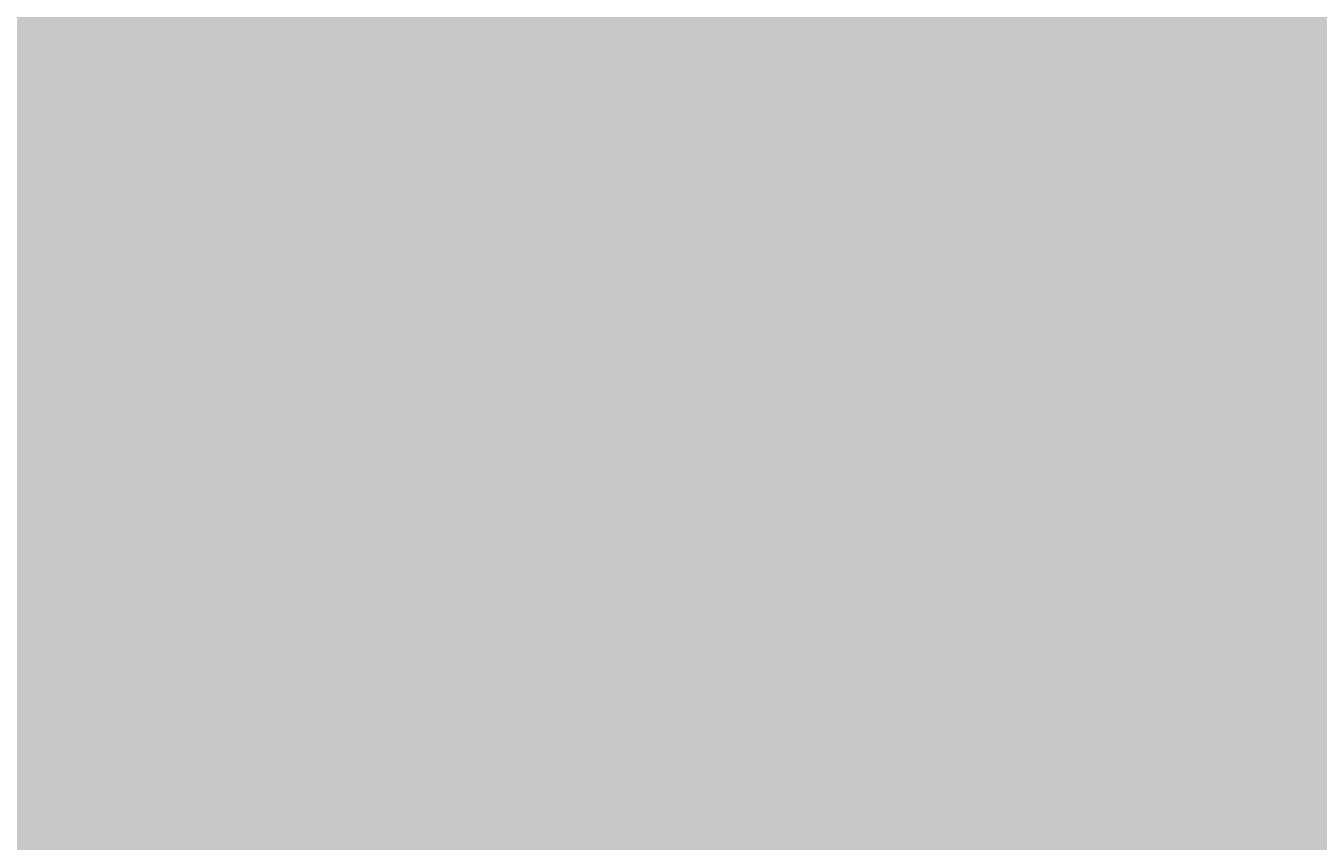
# Model space of a CAD drawing. Units: inches. Extents: x 84 to 1044, y -280 to 906.
# Tile 72 of 105: x 705 to 733, y 432 to 450. Entities that reach past the tile are written whole.
import ezdxf

# ---------------------------------------------------------------- set-up
doc = ezdxf.new("R2010")
doc.units = ezdxf.units.IN
doc.layers.add('A-ANNO-DIMS', color=2, linetype='Continuous', lineweight=18)
doc.layers.add('L-PLNT-PATT', color=9, linetype='Continuous', lineweight=9, true_color=0xafd9aa)
doc.styles.get("Standard").update_dxf_attribs({"font": 'arial.ttf'})
doc.dimstyles.get("Standard").update_dxf_attribs({"dimtxt": 0.18, "dimasz": 0.18, "dimexe": 0.18, "dimexo": 0.0625, "dimgap": 0.09, "dimtad": 0, "dimtih": 1, "dimtoh": 1, "dimdec": 4, "dimzin": 0, "dimdsep": 46, "dimtxsty": 'Standard', "dimcen": 0.09, "dimadec": 0, "dimazin": 0, "dimtfac": 1, "dimtdec": 4, "dimtofl": 0, "dimtmove": 0, "dimatfit": 3, "dimfxl": 1, "dimtolj": 1, "dimtzin": 0, "dimarcsym": 0})

# ---------------------------------------------------------------- blocks, each defined once
blk = doc.blocks.new('*D62')
at = {"layer": 'A-ANNO-DIMS', "color": 0, "lineweight": -2, "transparency": 16777216}
for p, q in [((203.179, 709.183), (203.179, 905.9)), ((203.359, 905.72), (549.232, 905.72)), ((895.894, 905.72), (550.021, 905.72)), ((896.074, 400.183), (896.074, 905.9))]:
    blk.add_line(p, q, dxfattribs=at)
at = {"layer": 'A-ANNO-DIMS', "color": 0, "transparency": 16777216}
for points in [[(203.359, 905.75), (203.359, 905.69), (203.179, 905.72)], [(895.894, 905.75), (895.894, 905.69), (896.074, 905.72)]]:
    blk.add_solid(points, dxfattribs=at)
at = {"layer": 'Defpoints', "color": 0, "transparency": 16777216}
for p in [(896.074, 905.72), (203.179, 709.12), (896.074, 400.12)]:
    blk.add_point(p, dxfattribs=at)
at = {"layer": 'A-ANNO-DIMS', "color": 0, "transparency": 16777216, "insert": (549.627, 905.72), "char_height": 0.18, "attachment_point": 5}
blk.add_mtext('\\A1;692.9', dxfattribs=at)

msp = doc.modelspace()

# ---------------------------------------------------------------- hatches: boundary and pattern name
at = {"layer": 'L-PLNT-PATT', "transparency": 33554597}
h = msp.add_hatch(color=256, dxfattribs=at)
h.dxf.hatch_style = 1
h.paths.add_polyline_path([(896.074, 511.12), (704.074, 511.12), (704.074, 491.62), (704.074, 419.62), (704.074, 400.12), (833.074, 400.12), (896.074, 400.12)])

# ---------------------------------------------------------------- dimensions: what is measured, and where the dimension line sits
at = {"layer": 'A-ANNO-DIMS'}
dim = msp.add_linear_dim(base=(896.074, 905.72), p1=(203.179, 709.12), p2=(896.074, 400.12), dimstyle='Standard', override={"dimdec": 1, "dimlfac": 1, "dimrnd": 0, "dimzin": 0, "dimdsep": 46, "dimlunit": 2}, dxfattribs=at)
dim.commit()
dim.dimension.update_dxf_attribs({"geometry": '*D62', "text_midpoint": (549.627, 905.72)})

doc.saveas('drawing.dxf')
